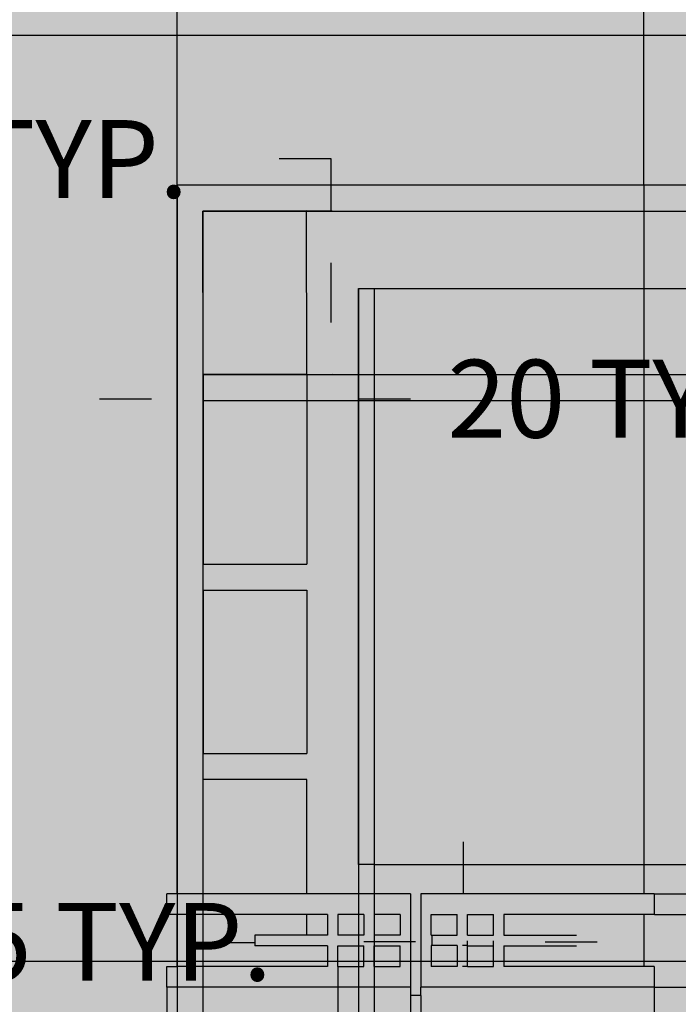
# Model space of a CAD drawing. Units: millimetres. Extents: x 131 to 845, y -20 to 1043.
# Tile 7 of 11: x 495 to 622, y 302 to 492. Entities that reach past the tile are written whole.
import ezdxf

# ---------------------------------------------------------------- set-up
doc = ezdxf.new("R2010")
doc.units = ezdxf.units.MM
doc.header["$MEASUREMENT"] = 0
for name, color, linetype, lineweight in [('A-ANNO-DIMS', 2, 'Continuous', 18), ('A-DOOR', 3, 'Continuous', 25), ('A-DOOR-PATT', 45, 'Continuous', 13), ('A-ELEV', 7, 'Continuous', 25), ('A-ELEV-PATT', 7, 'Continuous', 13), ('A-FLOR-HRAL', 6, 'Continuous', 25), ('A-WALL-PATT', 131, 'Continuous', 13)]:
    doc.layers.add(name, color=color, linetype=linetype, lineweight=lineweight)
doc.styles.get("Standard").update_dxf_attribs({"font": 'arial.ttf'})
doc.dimstyles.get("Standard").update_dxf_attribs({"dimtxt": 15, "dimasz": 10, "dimexe": 0.18, "dimexo": 0.0625, "dimgap": 5, "dimtad": 0, "dimtih": 1, "dimtoh": 1, "dimdec": 0, "dimzin": 0, "dimdsep": 46, "dimtxsty": 'Standard', "dimcen": 5, "dimadec": 0, "dimazin": 0, "dimtfac": 1, "dimtdec": 0, "dimtofl": 0, "dimtmove": 0, "dimatfit": 3, "dimfxl": 1, "dimtolj": 1, "dimtzin": 0, "dimarcsym": 0})

# ---------------------------------------------------------------- blocks, each defined once
blk = doc.blocks.new('RAIL-PANEL')
for p, q in [((5, 4), (0, 4)), ((0, 4), (0, 0)), ((5, 4), (5, 0)), ((5, 0), (0, 0))]:
    blk.add_line(p, q)
blk = doc.blocks.new('DOOR-GLASS-PANE')
for p, q in [((0, 0), (0, 31.5)), ((20, 31.5), (0, 31.5)), ((20, 0), (20, 31.5)), ((20, 0), (0, 0))]:
    blk.add_line(p, q)
blk = doc.blocks.new('*D9')
at = {"layer": 'A-ANNO-DIMS', "color": 0, "lineweight": -2, "transparency": 16777216}
for p, q in [((571.05, 313.91), (561.05, 313.91)), ((581.05, 313.22), (581.05, 314.09)), ((586.05, 313.22), (586.05, 314.09)), ((596.05, 313.91), (606.05, 313.91))]:
    blk.add_line(p, q, dxfattribs=at)
at = {"layer": 'A-ANNO-DIMS', "color": 0, "transparency": 16777216}
for points in [[(571.05, 315.58), (571.05, 312.24), (581.05, 313.91)], [(596.05, 315.58), (596.05, 312.24), (586.05, 313.91)]]:
    blk.add_solid(points, dxfattribs=at)
at = {"layer": 'Defpoints', "color": 0, "transparency": 16777216}
for p in [(581.05, 313.91), (581.05, 313.16), (586.05, 313.16)]:
    blk.add_point(p, dxfattribs=at)
at = {"layer": 'A-ANNO-DIMS', "color": 0, "transparency": 16777216, "insert": (409.24, 313.91), "char_height": 15, "attachment_point": 5}
blk.add_mtext('\\A1;BALCONY RAIL PANEL 5 TYP.', dxfattribs=at)
blk = doc.blocks.new('*D10')
at = {"layer": 'A-ANNO-DIMS', "color": 0, "lineweight": -2, "transparency": 16777216}
for p, q in [((580.3, 323.16), (580.3, 333.16)), ((580.98, 313.16), (580.12, 313.16)), ((580.98, 309.16), (580.12, 309.16)), ((580.3, 299.16), (580.3, 289.16)), ((580.3, 289.16), (570.3, 289.16))]:
    blk.add_line(p, q, dxfattribs=at)
at = {"layer": 'A-ANNO-DIMS', "color": 0, "transparency": 16777216}
for points in [[(578.63, 323.16), (581.96, 323.16), (580.3, 313.16)], [(578.63, 299.16), (581.96, 299.16), (580.3, 309.16)]]:
    blk.add_solid(points, dxfattribs=at)
at = {"layer": 'Defpoints', "color": 0, "transparency": 16777216}
for p in [(581.05, 313.16), (580.3, 309.16), (581.05, 309.16)]:
    blk.add_point(p, dxfattribs=at)
at = {"layer": 'A-ANNO-DIMS', "color": 0, "transparency": 16777216, "insert": (534.31, 289.16), "char_height": 15, "attachment_point": 5}
blk.add_mtext('\\A1;4 TYP.', dxfattribs=at)
blk = doc.blocks.new('*D11')
at = {"layer": 'A-ANNO-DIMS', "color": 0, "lineweight": -2, "transparency": 16777216}
for p, q in [((554.73, 464.78), (544.73, 464.78)), ((554.75, 454.78), (554.73, 464.78)), ((550.09, 454.77), (554.93, 454.78)), ((554.78, 433.28), (554.76, 444.78)), ((550.13, 423.27), (554.97, 423.28))]:
    blk.add_line(p, q, dxfattribs=at)
at = {"layer": 'A-ANNO-DIMS', "color": 0, "transparency": 16777216}
for points in [[(556.43, 444.78), (553.1, 444.77), (554.75, 454.78)], [(556.45, 433.28), (553.11, 433.27), (554.79, 423.28)]]:
    blk.add_solid(points, dxfattribs=at)
at = {"layer": 'Defpoints', "color": 0, "transparency": 16777216}
for p in [(550.02, 454.77), (554.75, 454.78), (550.07, 423.27)]:
    blk.add_point(p, dxfattribs=at)
at = {"layer": 'A-ANNO-DIMS', "color": 0, "transparency": 16777216, "insert": (399.96, 464.78), "char_height": 15, "attachment_point": 5}
blk.add_mtext('\\A1;DOOR GLASS PANE 32 TYP.', dxfattribs=at)
blk = doc.blocks.new('*D12')
at = {"layer": 'A-ANNO-DIMS', "color": 0, "lineweight": -2, "transparency": 16777216}
for p, q in [((530.07, 423.18), (530.08, 418.34)), ((550.07, 423.21), (550.08, 418.36)), ((520.08, 418.5), (510.08, 418.49)), ((560.08, 418.56), (570.08, 418.57))]:
    blk.add_line(p, q, dxfattribs=at)
at = {"layer": 'A-ANNO-DIMS', "color": 0, "transparency": 16777216}
for points in [[(520.07, 420.17), (520.08, 416.83), (530.08, 418.52)], [(560.07, 420.22), (560.08, 416.89), (550.08, 418.54)]]:
    blk.add_solid(points, dxfattribs=at)
at = {"layer": 'Defpoints', "color": 0, "transparency": 16777216}
for p in [(530.07, 423.24), (550.07, 423.27), (550.08, 418.54)]:
    blk.add_point(p, dxfattribs=at)
at = {"layer": 'A-ANNO-DIMS', "color": 0, "transparency": 16777216, "insert": (611.71, 418.57), "char_height": 15, "attachment_point": 5}
blk.add_mtext('\\A1;20 TYP.', dxfattribs=at)
blk = doc.blocks.new('*D50')
at = {"layer": 'A-ANNO-DIMS', "color": 0, "lineweight": -2, "transparency": 16777216}
for p, q in [((720.6, 488.6), (768.56, 488.6)), ((768.38, 478.6), (768.38, 287.12)), ((768.38, 70.31), (768.38, 261.79)), ((216.3, 60.31), (768.56, 60.31))]:
    blk.add_line(p, q, dxfattribs=at)
at = {"layer": 'A-ANNO-DIMS', "color": 0, "transparency": 16777216}
for points in [[(766.72, 478.6), (770.05, 478.6), (768.38, 488.6)], [(766.72, 70.31), (770.05, 70.31), (768.38, 60.31)]]:
    blk.add_solid(points, dxfattribs=at)
at = {"layer": 'Defpoints', "color": 0, "transparency": 16777216}
for p in [(720.53, 488.6), (768.38, 488.6), (216.23, 60.31)]:
    blk.add_point(p, dxfattribs=at)
at = {"layer": 'A-ANNO-DIMS', "color": 0, "transparency": 16777216, "insert": (768.38, 274.45), "char_height": 15, "attachment_point": 5}
blk.add_mtext('\\A1;428.3', dxfattribs=at)
blk = doc.blocks.new('*D51')
at = {"layer": 'A-ANNO-DIMS', "color": 0, "lineweight": -2, "transparency": 16777216}
for p, q in [((658.81, 488.53), (658.81, -10.22)), ((628.88, 312.6), (628.88, -10.22)), ((618.88, -10.04), (608.88, -10.04)), ((668.81, -10.04), (678.81, -10.04))]:
    blk.add_line(p, q, dxfattribs=at)
at = {"layer": 'A-ANNO-DIMS', "color": 0, "transparency": 16777216}
for points in [[(618.88, -8.37), (618.88, -11.7), (628.88, -10.04)], [(668.81, -8.37), (668.81, -11.7), (658.81, -10.04)]]:
    blk.add_solid(points, dxfattribs=at)
at = {"layer": 'Defpoints', "color": 0, "transparency": 16777216}
for p in [(658.81, 488.6), (628.88, 312.66), (658.81, -10.04)]:
    blk.add_point(p, dxfattribs=at)
at = {"layer": 'A-ANNO-DIMS', "color": 0, "transparency": 16777216, "insert": (715.07, -10.04), "char_height": 15, "attachment_point": 5}
blk.add_mtext('\\A1;29.923', dxfattribs=at)
blk = doc.blocks.new('*D58')
at = {"layer": 'A-ANNO-DIMS', "color": 0, "lineweight": -2, "transparency": 16777216}
for p, q in [((525.05, 459.87), (525.05, 1033.7)), ((535.05, 1033.52), (554.33, 1033.52)), ((605.05, 1033.52), (585.76, 1033.52)), ((615.05, 459.87), (615.05, 1033.7))]:
    blk.add_line(p, q, dxfattribs=at)
at = {"layer": 'A-ANNO-DIMS', "color": 0, "transparency": 16777216}
for points in [[(535.05, 1035.18), (535.05, 1031.85), (525.05, 1033.52)], [(605.05, 1035.18), (605.05, 1031.85), (615.05, 1033.52)]]:
    blk.add_solid(points, dxfattribs=at)
at = {"layer": 'Defpoints', "color": 0, "transparency": 16777216}
for p in [(615.05, 1033.52), (525.05, 459.8), (615.05, 459.8)]:
    blk.add_point(p, dxfattribs=at)
at = {"layer": 'A-ANNO-DIMS', "color": 0, "transparency": 16777216, "insert": (570.05, 1033.52), "char_height": 15, "attachment_point": 5}
blk.add_mtext('\\A1;90', dxfattribs=at)
blk = doc.blocks.new('*D59')
at = {"layer": 'A-ANNO-DIMS', "color": 0, "lineweight": -2, "transparency": 16777216}
for p, q in [((615.11, 459.8), (768.56, 459.8)), ((768.38, 449.8), (768.38, 395.14)), ((768.38, 315.16), (768.38, 369.82)), ((617.11, 305.16), (768.56, 305.16))]:
    blk.add_line(p, q, dxfattribs=at)
at = {"layer": 'A-ANNO-DIMS', "color": 0, "transparency": 16777216}
for points in [[(766.72, 449.8), (770.05, 449.8), (768.38, 459.8)], [(766.72, 315.16), (770.05, 315.16), (768.38, 305.16)]]:
    blk.add_solid(points, dxfattribs=at)
at = {"layer": 'Defpoints', "color": 0, "transparency": 16777216}
for p in [(615.05, 459.8), (617.05, 305.16), (768.38, 305.16)]:
    blk.add_point(p, dxfattribs=at)
at = {"layer": 'A-ANNO-DIMS', "color": 0, "transparency": 16777216, "insert": (768.38, 382.48), "char_height": 15, "attachment_point": 5}
blk.add_mtext('\\A1;154.65', dxfattribs=at)
blk = doc.blocks.new('*D60')
at = {"layer": 'A-ANNO-DIMS', "color": 0, "lineweight": -2, "transparency": 16777216}
for p, q in [((768.38, 333.16), (768.38, 343.16)), ((768.38, 343.16), (778.38, 343.16)), ((617.11, 323.16), (768.56, 323.16)), ((617.11, 305.16), (768.56, 305.16)), ((768.38, 295.16), (768.38, 285.16))]:
    blk.add_line(p, q, dxfattribs=at)
at = {"layer": 'A-ANNO-DIMS', "color": 0, "transparency": 16777216}
for points in [[(766.72, 333.16), (770.05, 333.16), (768.38, 323.16)], [(766.72, 295.16), (770.05, 295.16), (768.38, 305.16)]]:
    blk.add_solid(points, dxfattribs=at)
at = {"layer": 'Defpoints', "color": 0, "transparency": 16777216}
for p in [(617.05, 323.16), (768.38, 323.16), (617.05, 305.16)]:
    blk.add_point(p, dxfattribs=at)
at = {"layer": 'A-ANNO-DIMS', "color": 0, "transparency": 16777216, "insert": (793.44, 343.16), "char_height": 15, "attachment_point": 5}
blk.add_mtext('\\A1;18', dxfattribs=at)
blk = doc.blocks.new('*D61')
at = {"layer": 'A-ANNO-DIMS', "color": 0, "lineweight": -2, "transparency": 16777216}
for p, q in [((768.38, 333.16), (768.38, 343.16)), ((768.38, 343.16), (778.38, 343.16)), ((617.11, 323.16), (768.56, 323.16)), ((617.11, 319.16), (768.56, 319.16)), ((768.38, 309.16), (768.38, 299.16))]:
    blk.add_line(p, q, dxfattribs=at)
at = {"layer": 'A-ANNO-DIMS', "color": 0, "transparency": 16777216}
for points in [[(766.72, 333.16), (770.05, 333.16), (768.38, 323.16)], [(766.72, 309.16), (770.05, 309.16), (768.38, 319.16)]]:
    blk.add_solid(points, dxfattribs=at)
at = {"layer": 'Defpoints', "color": 0, "transparency": 16777216}
for p in [(617.05, 323.16), (768.38, 323.16), (617.05, 319.16)]:
    blk.add_point(p, dxfattribs=at)
at = {"layer": 'A-ANNO-DIMS', "color": 0, "transparency": 16777216, "insert": (788.57, 343.16), "char_height": 15, "attachment_point": 5}
blk.add_mtext('\\A1;4', dxfattribs=at)
blk = doc.blocks.new('*D62')
at = {"layer": 'A-ANNO-DIMS', "color": 0, "lineweight": -2, "transparency": 16777216}
for p, q in [((525.05, 459.74), (525.05, -10.22)), ((530.02, 454.68), (530.02, -10.22)), ((515.05, -10.04), (505.05, -10.04)), ((540.02, -10.04), (550.02, -10.04))]:
    blk.add_line(p, q, dxfattribs=at)
at = {"layer": 'A-ANNO-DIMS', "color": 0, "transparency": 16777216}
for points in [[(515.05, -8.37), (515.05, -11.7), (525.05, -10.04)], [(540.02, -8.37), (540.02, -11.7), (530.02, -10.04)]]:
    blk.add_solid(points, dxfattribs=at)
at = {"layer": 'Defpoints', "color": 0, "transparency": 16777216}
for p in [(525.05, 459.8), (530.02, 454.74), (530.02, -10.04)]:
    blk.add_point(p, dxfattribs=at)
at = {"layer": 'A-ANNO-DIMS', "color": 0, "transparency": 16777216, "insert": (580.63, -10.04), "char_height": 15, "attachment_point": 5}
blk.add_mtext('\\A1;4.977', dxfattribs=at)
blk = doc.blocks.new('*D63')
at = {"layer": 'A-ANNO-DIMS', "color": 0, "lineweight": -2, "transparency": 16777216}
for p, q in [((768.38, 469.8), (768.38, 479.8)), ((768.38, 479.8), (778.38, 479.8)), ((525.11, 459.8), (768.56, 459.8)), ((530.09, 454.74), (768.56, 454.74)), ((768.38, 444.74), (768.38, 434.74))]:
    blk.add_line(p, q, dxfattribs=at)
at = {"layer": 'A-ANNO-DIMS', "color": 0, "transparency": 16777216}
for points in [[(766.72, 469.8), (770.05, 469.8), (768.38, 459.8)], [(766.72, 444.74), (770.05, 444.74), (768.38, 454.74)]]:
    blk.add_solid(points, dxfattribs=at)
at = {"layer": 'Defpoints', "color": 0, "transparency": 16777216}
for p in [(525.05, 459.8), (768.38, 459.8), (530.02, 454.74)]:
    blk.add_point(p, dxfattribs=at)
at = {"layer": 'A-ANNO-DIMS', "color": 0, "transparency": 16777216, "insert": (808.75, 479.8), "char_height": 15, "attachment_point": 5}
blk.add_mtext('\\A1;5.065', dxfattribs=at)
blk = doc.blocks.new('*D64')
at = {"layer": 'A-ANNO-DIMS', "color": 0, "lineweight": -2, "transparency": 16777216}
for p, q in [((768.38, 433.24), (768.38, 443.24)), ((768.38, 443.24), (778.38, 443.24)), ((530.13, 423.24), (768.56, 423.24)), ((530.11, 418.2), (768.56, 418.2)), ((768.38, 408.2), (768.38, 398.2))]:
    blk.add_line(p, q, dxfattribs=at)
at = {"layer": 'A-ANNO-DIMS', "color": 0, "transparency": 16777216}
for points in [[(766.72, 433.24), (770.05, 433.24), (768.38, 423.24)], [(766.72, 408.2), (770.05, 408.2), (768.38, 418.2)]]:
    blk.add_solid(points, dxfattribs=at)
at = {"layer": 'Defpoints', "color": 0, "transparency": 16777216}
for p in [(530.07, 423.24), (768.38, 423.24), (530.05, 418.2)]:
    blk.add_point(p, dxfattribs=at)
at = {"layer": 'A-ANNO-DIMS', "color": 0, "transparency": 16777216, "insert": (808.69, 443.24), "char_height": 15, "attachment_point": 5}
blk.add_mtext('\\A1;5.036', dxfattribs=at)
blk = doc.blocks.new('*D65')
at = {"layer": 'A-ANNO-DIMS', "color": 0, "lineweight": -2, "transparency": 16777216}
for p, q in [((560.05, 439.74), (560.05, -10.22)), ((563.05, 439.74), (563.05, -10.22)), ((550.05, -10.04), (540.05, -10.04)), ((573.05, -10.04), (583.05, -10.04))]:
    blk.add_line(p, q, dxfattribs=at)
at = {"layer": 'A-ANNO-DIMS', "color": 0, "transparency": 16777216}
for points in [[(550.05, -8.37), (550.05, -11.7), (560.05, -10.04)], [(573.05, -8.37), (573.05, -11.7), (563.05, -10.04)]]:
    blk.add_solid(points, dxfattribs=at)
at = {"layer": 'Defpoints', "color": 0, "transparency": 16777216}
for p in [(560.05, 439.8), (563.05, 439.8), (563.05, -10.04)]:
    blk.add_point(p, dxfattribs=at)
at = {"layer": 'A-ANNO-DIMS', "color": 0, "transparency": 16777216, "insert": (592.96, -10.04), "char_height": 15, "attachment_point": 5}
blk.add_mtext('\\A1;3', dxfattribs=at)
blk = doc.blocks.new('*D66')
at = {"layer": 'A-ANNO-DIMS', "color": 0, "lineweight": -2, "transparency": 16777216}
for p, q in [((563.11, 439.8), (768.56, 439.8)), ((768.38, 429.8), (768.38, 396.84)), ((768.38, 338.8), (768.38, 371.77)), ((563.11, 328.8), (768.56, 328.8))]:
    blk.add_line(p, q, dxfattribs=at)
at = {"layer": 'A-ANNO-DIMS', "color": 0, "transparency": 16777216}
for points in [[(766.72, 429.8), (770.05, 429.8), (768.38, 439.8)], [(766.72, 338.8), (770.05, 338.8), (768.38, 328.8)]]:
    blk.add_solid(points, dxfattribs=at)
at = {"layer": 'Defpoints', "color": 0, "transparency": 16777216}
for p in [(563.05, 439.8), (768.38, 439.8), (563.05, 328.8)]:
    blk.add_point(p, dxfattribs=at)
at = {"layer": 'A-ANNO-DIMS', "color": 0, "transparency": 16777216, "insert": (768.38, 384.3), "char_height": 15, "attachment_point": 5}
blk.add_mtext('\\A1;111', dxfattribs=at)
blk = doc.blocks.new('*D67')
at = {"layer": 'A-ANNO-DIMS', "color": 0, "lineweight": -2, "transparency": 16777216}
for p, q in [((525.05, 459.74), (525.05, -10.22)), ((560.05, 439.74), (560.05, -10.22)), ((515.05, -10.04), (505.05, -10.04)), ((570.05, -10.04), (580.05, -10.04))]:
    blk.add_line(p, q, dxfattribs=at)
at = {"layer": 'A-ANNO-DIMS', "color": 0, "transparency": 16777216}
for points in [[(515.05, -8.37), (515.05, -11.7), (525.05, -10.04)], [(570.05, -8.37), (570.05, -11.7), (560.05, -10.04)]]:
    blk.add_solid(points, dxfattribs=at)
at = {"layer": 'Defpoints', "color": 0, "transparency": 16777216}
for p in [(525.05, 459.8), (560.05, 439.8), (560.05, -10.04)]:
    blk.add_point(p, dxfattribs=at)
at = {"layer": 'A-ANNO-DIMS', "color": 0, "transparency": 16777216, "insert": (542.55, -10.04), "char_height": 15, "attachment_point": 5}
blk.add_mtext('\\A1;35', dxfattribs=at)
blk = doc.blocks.new('*D68')
at = {"layer": 'A-ANNO-DIMS', "color": 0, "lineweight": -2, "transparency": 16777216}
for p, q in [((523.05, 305.1), (523.05, -10.22)), ((617.05, 305.1), (617.05, -10.22)), ((533.05, -10.04), (554.33, -10.04)), ((607.05, -10.04), (585.76, -10.04))]:
    blk.add_line(p, q, dxfattribs=at)
at = {"layer": 'A-ANNO-DIMS', "color": 0, "transparency": 16777216}
for points in [[(533.05, -8.37), (533.05, -11.7), (523.05, -10.04)], [(607.05, -8.37), (607.05, -11.7), (617.05, -10.04)]]:
    blk.add_solid(points, dxfattribs=at)
at = {"layer": 'Defpoints', "color": 0, "transparency": 16777216}
for p in [(523.05, 305.16), (617.05, 305.16), (617.05, -10.04)]:
    blk.add_point(p, dxfattribs=at)
at = {"layer": 'A-ANNO-DIMS', "color": 0, "transparency": 16777216, "insert": (570.05, -10.04), "char_height": 15, "attachment_point": 5}
blk.add_mtext('\\A1;94', dxfattribs=at)
blk = doc.blocks.new('*D69')
at = {"layer": 'A-ANNO-DIMS', "color": 0, "lineweight": -2, "transparency": 16777216}
for p, q in [((570.05, 303.56), (570.05, -10.22)), ((572.05, 303.56), (572.05, -10.22)), ((560.05, -10.04), (550.05, -10.04)), ((582.05, -10.04), (592.05, -10.04))]:
    blk.add_line(p, q, dxfattribs=at)
at = {"layer": 'A-ANNO-DIMS', "color": 0, "transparency": 16777216}
for points in [[(560.05, -8.37), (560.05, -11.7), (570.05, -10.04)], [(582.05, -8.37), (582.05, -11.7), (572.05, -10.04)]]:
    blk.add_solid(points, dxfattribs=at)
at = {"layer": 'Defpoints', "color": 0, "transparency": 16777216}
for p in [(570.05, 303.62), (572.05, 303.62), (572.05, -10.04)]:
    blk.add_point(p, dxfattribs=at)
at = {"layer": 'A-ANNO-DIMS', "color": 0, "transparency": 16777216, "insert": (616.63, -10.04), "char_height": 15, "attachment_point": 5}
blk.add_mtext('\\A1;2.00', dxfattribs=at)
blk = doc.blocks.new('*D70')
at = {"layer": 'A-ANNO-DIMS', "color": 0, "lineweight": -2, "transparency": 16777216}
for p, q in [((556.05, 309.1), (556.05, -10.22)), ((523.05, 305.1), (523.05, -10.22)), ((513.05, -10.04), (503.05, -10.04)), ((566.05, -10.04), (576.05, -10.04))]:
    blk.add_line(p, q, dxfattribs=at)
at = {"layer": 'A-ANNO-DIMS', "color": 0, "transparency": 16777216}
for points in [[(513.05, -8.37), (513.05, -11.7), (523.05, -10.04)], [(566.05, -8.37), (566.05, -11.7), (556.05, -10.04)]]:
    blk.add_solid(points, dxfattribs=at)
at = {"layer": 'Defpoints', "color": 0, "transparency": 16777216}
for p in [(556.05, 309.16), (523.05, 305.16), (556.05, -10.04)]:
    blk.add_point(p, dxfattribs=at)
at = {"layer": 'A-ANNO-DIMS', "color": 0, "transparency": 16777216, "insert": (539.55, -10.04), "char_height": 15, "attachment_point": 5}
blk.add_mtext('\\A1;33', dxfattribs=at)
blk = doc.blocks.new('*D71')
at = {"layer": 'A-ANNO-DIMS', "color": 0, "lineweight": -2, "transparency": 16777216}
for p, q in [((556.05, 309.1), (556.05, -10.22)), ((563.05, 309.1), (563.05, -10.22)), ((546.05, -10.04), (536.05, -10.04)), ((573.05, -10.04), (583.05, -10.04))]:
    blk.add_line(p, q, dxfattribs=at)
at = {"layer": 'A-ANNO-DIMS', "color": 0, "transparency": 16777216}
for points in [[(546.05, -8.37), (546.05, -11.7), (556.05, -10.04)], [(573.05, -8.37), (573.05, -11.7), (563.05, -10.04)]]:
    blk.add_solid(points, dxfattribs=at)
at = {"layer": 'Defpoints', "color": 0, "transparency": 16777216}
for p in [(556.05, 309.16), (563.05, 309.16), (563.05, -10.04)]:
    blk.add_point(p, dxfattribs=at)
at = {"layer": 'A-ANNO-DIMS', "color": 0, "transparency": 16777216, "insert": (592.9, -10.04), "char_height": 15, "attachment_point": 5}
blk.add_mtext('\\A1;7', dxfattribs=at)
blk = doc.blocks.new('*D75')
at = {"layer": 'A-ANNO-DIMS', "color": 0, "lineweight": -2, "transparency": 16777216}
for p, q in [((462.24, 1033.52), (452.24, 1033.52)), ((472.24, 310.22), (472.24, 1033.7)), ((489.56, 300.22), (489.56, 1033.7)), ((499.56, 1033.52), (509.56, 1033.52))]:
    blk.add_line(p, q, dxfattribs=at)
at = {"layer": 'A-ANNO-DIMS', "color": 0, "transparency": 16777216}
for points in [[(462.24, 1035.18), (462.24, 1031.85), (472.24, 1033.52)], [(499.56, 1035.18), (499.56, 1031.85), (489.56, 1033.52)]]:
    blk.add_solid(points, dxfattribs=at)
at = {"layer": 'Defpoints', "color": 0, "transparency": 16777216}
for p in [(489.56, 1033.52), (472.24, 310.16), (489.56, 300.16)]:
    blk.add_point(p, dxfattribs=at)
at = {"layer": 'A-ANNO-DIMS', "color": 0, "transparency": 16777216, "insert": (539.08, 1033.52), "char_height": 15, "attachment_point": 5}
blk.add_mtext('\\A1;17.32', dxfattribs=at)
blk = doc.blocks.new('*D76')
at = {"layer": 'A-ANNO-DIMS', "color": 0, "lineweight": -2, "transparency": 16777216}
for p, q in [((768.38, 320.16), (768.38, 330.16)), ((472.3, 310.16), (768.56, 310.16)), ((489.62, 300.16), (768.56, 300.16)), ((768.38, 290.16), (768.38, 280.16)), ((768.38, 280.16), (758.38, 280.16))]:
    blk.add_line(p, q, dxfattribs=at)
at = {"layer": 'A-ANNO-DIMS', "color": 0, "transparency": 16777216}
for points in [[(766.72, 320.16), (770.05, 320.16), (768.38, 310.16)], [(766.72, 290.16), (770.05, 290.16), (768.38, 300.16)]]:
    blk.add_solid(points, dxfattribs=at)
at = {"layer": 'Defpoints', "color": 0, "transparency": 16777216}
for p in [(472.24, 310.16), (489.56, 300.16), (768.38, 300.16)]:
    blk.add_point(p, dxfattribs=at)
at = {"layer": 'A-ANNO-DIMS', "color": 0, "transparency": 16777216, "insert": (743.37, 280.16), "char_height": 15, "attachment_point": 5}
blk.add_mtext('\\A1;10', dxfattribs=at)
blk = doc.blocks.new('*D85')
at = {"layer": 'A-ANNO-DIMS', "color": 0, "lineweight": -2, "transparency": 16777216}
for p, q in [((768.38, 301.78), (768.38, 311.78)), ((768.38, 311.78), (778.38, 311.78)), ((639.93, 291.78), (768.56, 291.78)), ((602.06, 283.26), (768.56, 283.26)), ((768.38, 273.26), (768.38, 263.26))]:
    blk.add_line(p, q, dxfattribs=at)
at = {"layer": 'A-ANNO-DIMS', "color": 0, "transparency": 16777216}
for points in [[(766.72, 301.78), (770.05, 301.78), (768.38, 291.78)], [(766.72, 273.26), (770.05, 273.26), (768.38, 283.26)]]:
    blk.add_solid(points, dxfattribs=at)
at = {"layer": 'Defpoints', "color": 0, "transparency": 16777216}
for p in [(639.87, 291.78), (768.38, 291.78), (601.99, 283.26)]:
    blk.add_point(p, dxfattribs=at)
at = {"layer": 'A-ANNO-DIMS', "color": 0, "transparency": 16777216, "insert": (808.63, 311.78), "char_height": 15, "attachment_point": 5}
blk.add_mtext('\\A1;8.522', dxfattribs=at)

msp = doc.modelspace()

# ---------------------------------------------------------------- hatches: boundary and pattern name
at = {"layer": 'A-DOOR-PATT'}
h = msp.add_hatch(color=256, dxfattribs=at)
h.dxf.hatch_style = 1
h.paths.add_polyline_path([(615.0467, 459.8046), (525.0467, 459.8046), (525.0467, 323.1596), (530.0467, 323.1596), (530.0467, 345.2044), (550.0467, 345.2044), (550.0467, 323.1596), (570.0467, 323.1596), (570.0467, 305.1596), (570.0467, 303.6234), (572.0453, 303.6234), (572.0467, 305.1596), (572.0467, 323.1596), (615.0467, 323.1596)])
h.paths.add_polyline_path([(563.0467, 328.8046), (560.0467, 328.8046), (560.0467, 439.8046), (563.0467, 439.8046)], flags=16)
h.paths.add_polyline_path([(550.0467, 386.7044), (530.0467, 386.7044), (530.0467, 418.2044), (550.0467, 418.2044)], flags=16)
h.paths.add_polyline_path([(550.0467, 381.7044), (550.0467, 350.2044), (530.0467, 350.2044), (530.0467, 381.7044)], flags=16)
h.paths.add_polyline_path([(550.0467, 423.2044), (530.0467, 423.2044), (530.0467, 454.8046), (550.0467, 454.8046)], flags=16)
h.paths.add_polyline_path([(615.0467, 693.2667), (525.0467, 693.2667), (525.0467, 542.1664), (615.0467, 542.1664)])
h.paths.add_polyline_path([(563.0467, 562.2667), (560.0467, 562.2667), (560.0467, 673.2667), (563.0467, 673.2667)], flags=16)
h.paths.add_polyline_path([(550.0467, 583.6664), (530.0467, 583.6664), (530.0467, 615.1664), (550.0467, 615.1664)], flags=16)
h.paths.add_polyline_path([(550.0467, 578.6664), (550.0467, 547.1664), (530.0467, 547.1664), (530.0467, 578.6664)], flags=16)
h.paths.add_polyline_path([(550.0467, 620.1664), (530.0467, 620.1664), (530.0467, 651.6664), (550.0467, 651.6664)], flags=16)
h.paths.add_polyline_path([(550.0467, 656.6664), (530.0467, 656.6664), (530.0467, 688.2667), (550.0467, 688.2667)], flags=16)
h = msp.add_hatch(color=256, dxfattribs=at)
h.dxf.hatch_style = 1
h.paths.add_polyline_path([(523.0467, 323.1596), (523.0467, 319.1596), (525.0467, 319.1596), (554.0467, 319.1596), (554.0467, 315.1596), (540.0467, 315.1596), (540.0467, 313.1596), (554.0467, 313.1596), (554.0467, 309.1596), (525.0467, 309.1596), (523.0467, 309.1596), (523.0467, 305.1596), (525.0467, 305.1596), (570.0467, 305.1596), (570.0467, 323.1596)])
h.paths.add_polyline_path([(556.0467, 319.1596), (561.0467, 319.1596), (561.0467, 315.1596), (556.0467, 315.1596)], flags=16)
h.paths.add_polyline_path([(556.0467, 313.1596), (561.0467, 313.1596), (561.0467, 309.1596), (556.0467, 309.1596)], flags=16)
h.paths.add_polyline_path([(563.0467, 319.1596), (568.0467, 319.1596), (568.0467, 315.1596), (563.0467, 315.1596)], flags=16)
h.paths.add_polyline_path([(563.0467, 313.1596), (568.0467, 313.1596), (568.0467, 309.1596), (563.0467, 309.1596)], flags=16)
h.paths.add_polyline_path([(572.0467, 323.1596), (572.0467, 305.1596), (617.0467, 305.1596), (617.0467, 309.1596), (588.0467, 309.1596), (588.0467, 313.1596), (602.0467, 313.1596), (602.0467, 315.1596), (588.0467, 315.1596), (588.0467, 319.1596), (617.0467, 319.1596), (617.0467, 323.1596)])
h.paths.add_polyline_path([(581.0467, 319.1596), (586.0467, 319.1596), (586.0467, 315.1596), (581.0467, 315.1596)], flags=16)
h.paths.add_polyline_path([(579.0467, 319.1596), (579.0467, 315.1596), (574.0467, 315.1596), (574.0467, 319.1596)], flags=16)
h.paths.add_polyline_path([(581.0467, 313.1596), (586.0467, 313.1596), (586.0467, 309.1596), (581.0467, 309.1596)], flags=16)
h.paths.add_polyline_path([(579.0467, 313.1596), (579.0467, 309.1596), (574.0467, 309.1596), (574.0467, 313.1596)], flags=16)
at = {"layer": 'A-ELEV-PATT', "transparency": 33554681}
h = msp.add_hatch(color=256, dxfattribs=at)
h.set_gradient(color1=(99, 100, 102), color2=(199, 200, 202), name='SPHERICAL')
h.paths.add_polyline_path([(550.0467, 688.2667), (530.0467, 688.2667), (530.0467, 656.6664), (550.0467, 656.6664)])
h.paths.add_polyline_path([(530.0467, 620.1664), (550.0467, 620.1664), (550.0467, 651.6664), (530.0467, 651.6664)])
h.paths.add_polyline_path([(550.0467, 615.1664), (530.0467, 615.1664), (530.0467, 583.6664), (550.0467, 583.6664)])
h.paths.add_polyline_path([(550.0467, 547.1664), (550.0467, 578.6664), (530.0467, 578.6664), (530.0467, 547.1664)])
h.paths.add_polyline_path([(563.0467, 673.2667), (560.0467, 673.2667), (560.0467, 562.2667), (563.0467, 562.2667)])
h.paths.add_polyline_path([(550.0467, 423.2044), (550.0467, 454.8046), (530.0467, 454.8046), (530.0467, 423.2044)])
h.paths.add_polyline_path([(550.0467, 418.2044), (530.0467, 418.2044), (530.0467, 386.7044), (550.0467, 386.7044)])
h.paths.add_polyline_path([(530.0467, 350.2044), (550.0467, 350.2044), (550.0467, 381.7044), (530.0467, 381.7044)])
h.paths.add_polyline_path([(550.0467, 323.1596), (550.0467, 345.2044), (530.0467, 345.2044), (530.0467, 323.1596)])
h.paths.add_polyline_path([(563.0467, 439.8046), (560.0467, 439.8046), (560.0467, 328.8046), (563.0467, 328.8046)])
h = msp.add_hatch(color=256, dxfattribs=at)
h.set_gradient(color1=(255, 255, 255), color2=(199, 200, 202), name='INVSPHERICAL')
h.paths.add_polyline_path([(459.5586, 310.1596), (472.2381, 310.1596), (489.5586, 300.1596), (650.5349, 300.1596), (628.8842, 312.6596), (628.8842, 488.5953), (459.5586, 488.5953)])
h.paths.add_polyline_path([(525.0467, 459.8046), (615.0467, 459.8046), (615.0467, 323.1596), (617.0467, 323.1596), (617.0467, 319.1596), (615.0467, 319.1596), (615.0467, 309.1596), (617.0467, 309.1596), (617.0467, 305.1596), (572.0467, 305.1596), (572.0453, 303.6234), (570.0467, 303.6234), (570.0467, 305.1596), (525.0467, 305.1596), (523.0467, 305.1596), (523.0467, 309.1596), (525.0467, 309.1596), (525.0467, 319.1596), (523.0467, 319.1596), (523.0467, 323.1596), (525.0467, 323.1596)], flags=16)
h.paths.add_polyline_path([(530.0467, 454.8046), (550.0467, 454.8046), (550.0467, 423.2044), (530.0467, 423.2044)], flags=0)
h.paths.add_polyline_path([(530.0467, 418.2044), (550.0467, 418.2044), (550.0467, 386.7044), (530.0467, 386.7044)], flags=0)
h.paths.add_polyline_path([(560.0467, 439.8046), (563.0467, 439.8046), (563.0467, 328.8046), (560.0467, 328.8046)], flags=0)
h.paths.add_polyline_path([(530.0467, 381.7044), (550.0467, 381.7044), (550.0467, 350.2044), (530.0467, 350.2044)], flags=0)
h.paths.add_polyline_path([(554.0467, 319.1596), (554.0467, 315.1596), (540.0467, 315.1596), (540.0467, 313.7044), (530.0467, 313.7044), (530.0467, 319.1596)], flags=0)
h.paths.add_polyline_path([(556.0467, 319.1596), (561.0467, 319.1596), (561.0467, 315.1596), (556.0467, 315.1596)], flags=0)
h.paths.add_polyline_path([(563.0467, 319.1596), (568.0467, 319.1596), (568.0467, 315.1596), (563.0467, 315.1596)], flags=0)
h.paths.add_polyline_path([(556.0467, 313.1596), (561.0467, 313.1596), (561.0467, 309.1596), (556.0467, 309.1596)], flags=0)
h.paths.add_polyline_path([(563.0467, 313.1596), (568.0467, 313.1596), (568.0467, 309.1596), (563.0467, 309.1596)], flags=0)
h.paths.add_polyline_path([(574.0467, 319.1596), (579.0467, 319.1596), (579.0467, 315.1596), (574.1854, 315.1596), (574.1854, 313.1596), (579.0467, 313.1596), (579.0467, 309.1596), (574.0467, 309.1596), (574.0467, 313.1596), (574.1854, 315.1596), (574.0467, 315.1596)], flags=0)
h.paths.add_polyline_path([(581.0467, 319.1596), (586.0467, 319.1596), (586.0467, 315.1596), (581.0467, 315.1596)], flags=0)
h.paths.add_polyline_path([(581.0467, 313.1596), (586.0467, 313.1596), (586.0467, 309.1596), (581.0467, 309.1596)], flags=0)
h = msp.add_hatch(color=256, dxfattribs=at)
h.set_gradient(color1=(79, 2, 22), color2=(98, 46, 19), name='SPHERICAL')
h.paths.add_polyline_path([(615.0467, 459.8046), (525.0467, 459.8046), (525.0467, 323.1596), (530.0467, 323.1596), (530.0467, 345.2044), (550.0467, 345.2044), (550.0467, 323.1596), (570.0467, 323.1596), (570.0467, 305.1596), (570.0467, 303.6234), (572.0453, 303.6234), (572.0467, 305.1596), (572.0467, 323.1596), (615.0467, 323.1596)])
h.paths.add_polyline_path([(563.0467, 328.8046), (560.0467, 328.8046), (560.0467, 439.8046), (563.0467, 439.8046)], flags=16)
h.paths.add_polyline_path([(550.0467, 386.7044), (530.0467, 386.7044), (530.0467, 418.2044), (550.0467, 418.2044)], flags=16)
h.paths.add_polyline_path([(550.0467, 381.7044), (550.0467, 350.2044), (530.0467, 350.2044), (530.0467, 381.7044)], flags=16)
h.paths.add_polyline_path([(550.0467, 423.2044), (530.0467, 423.2044), (530.0467, 454.8046), (550.0467, 454.8046)], flags=16)
h = msp.add_hatch(color=256, dxfattribs=at)
h.set_gradient(color1=(79, 2, 22), color2=(126, 16, 40), name='INVSPHERICAL')
h.paths.add_polyline_path([(615.0467, 309.1596), (615.0467, 319.1596), (617.0467, 319.1596), (617.0467, 323.1596), (572.0467, 323.1596), (572.0467, 305.1596), (617.0467, 305.1596), (617.0467, 309.1596)])
h.paths.add_polyline_path([(586.0467, 309.1596), (581.0467, 309.1596), (581.0467, 313.1596), (586.0467, 313.1596)], flags=16)
h.paths.add_polyline_path([(586.0467, 315.1596), (581.0467, 315.1596), (581.0467, 319.1596), (586.0467, 319.1596)], flags=16)
h.paths.add_polyline_path([(579.0467, 309.1596), (574.0467, 309.1596), (574.0467, 313.1596), (574.1854, 313.1596), (574.1854, 315.1596), (574.0467, 315.1596), (574.0467, 319.1596), (579.0467, 319.1596), (579.0467, 315.1596), (574.1854, 315.1596), (574.1854, 313.1596), (579.0467, 313.1596)], flags=16)
h = msp.add_hatch(color=256, dxfattribs=at)
h.set_gradient(color1=(79, 2, 22), color2=(126, 16, 40), name='INVSPHERICAL')
h.paths.add_polyline_path([(530.0467, 313.7044), (530.0467, 319.1596), (525.0467, 319.1596), (525.0467, 309.1596), (554.0467, 309.1596), (554.0467, 313.1596), (540.0467, 313.1596), (540.0467, 313.7044)])
at = {"layer": 'A-WALL-PATT'}
h = msp.add_hatch(color=256, dxfattribs=at)
h.dxf.hatch_style = 1
h.paths.add_polyline_path([(449.5586, 833.5953), (451.6297, 835.6663), (451.6297, 885.6663), (466.6297, 885.6663), (466.6297, 891.3345), (330.6595, 891.3345), (330.6595, 856.8345), (292.1595, 856.8345), (292.1595, 798.4332), (336.1595, 798.4332), (336.1595, 178.4332), (246.1595, 178.4332), (246.1595, 798.4332), (290.1595, 798.4332), (290.1595, 856.8345), (259.6595, 856.8345), (255.6595, 860.8345), (255.6595, 927.8345), (290.1595, 927.8345), (290.1595, 960.6663), (216.2327, 960.6663), (216.2327, 60.3131), (459.5586, 60.3131), (459.5586, 97.8131), (459.5586, 252.07), (459.5586, 283.5561), (369.5586, 283.5561), (369.5586, 763.5561), (439.5586, 763.5561), (439.5586, 778.6714), (439.5586, 793.5953), (439.5586, 796.5953), (441.5586, 798.5953), (444.5586, 798.5953), (444.5586, 813.5953), (444.5586, 816.5953), (446.5586, 818.5953), (449.5586, 818.5953)])
h.paths.add_polyline_path([(466.6297, 960.6663), (292.1595, 960.6663), (292.1595, 927.8345), (326.6595, 927.8345), (330.6595, 923.8345), (330.6595, 893.3345), (466.6297, 893.3345)], flags=17)
h.paths.add_polyline_path([(720.5349, 813.5953), (720.5349, 818.5953), (710.5349, 818.5953), (449.5586, 818.5953), (446.5586, 818.5953), (444.5586, 816.5953), (444.5586, 813.5953), (444.5586, 798.5953), (705.5349, 798.5953), (705.5349, 513.5953), (705.5349, 498.5953), (680.5349, 498.5953), (680.5349, 488.5953), (705.5349, 488.5953), (720.5349, 488.5953), (720.5349, 513.5953)])
h.paths.add_polyline_path([(680.5349, 498.5953), (412.6606, 498.5953), (412.6606, 488.5953), (680.5349, 488.5953)])

# ---------------------------------------------------------------- linework, layer by layer
at = {"layer": 'A-DOOR'}
for p, q in [((525.0467, 459.8046), (615.0467, 459.8046)), ((525.0467, 323.1596), (525.0467, 459.8046)), ((615.0467, 459.8046), (615.0467, 323.1596)), ((550.0467, 345.2044), (530.0467, 345.2044)), ((530.0467, 323.1596), (530.0467, 345.2044)), ((550.0467, 323.1596), (550.0467, 345.2044)), ((570.0467, 305.1596), (570.0467, 303.6234)), ((570.0467, 303.6234), (572.0453, 303.6234)), ((572.0453, 303.6234), (572.0467, 305.1596))]:
    msp.add_line(p, q, dxfattribs=at)
msp.add_lwpolyline([(560.0467, 439.8046), (563.0467, 439.8046), (563.0467, 328.8046), (560.0467, 328.8046)], close=True, dxfattribs=at)
at = {"layer": 'A-ELEV'}
msp.add_line((705.5349, 488.5953), (412.6606, 488.5953), dxfattribs=at)
at = {"layer": 'A-FLOR-HRAL'}
for p, q in [((523.0467, 319.1596), (523.0467, 323.1596)), ((570.0467, 323.1596), (523.0467, 323.1596)), ((570.0467, 323.1596), (570.0467, 305.1596)), ((617.0467, 323.1596), (572.0467, 323.1596)), ((572.0467, 323.1596), (572.0467, 305.1596)), ((617.0467, 323.1596), (617.0467, 319.1596)), ((525.0467, 319.1596), (523.0467, 319.1596)), ((525.0467, 309.1596), (525.0467, 319.1596)), ((554.0467, 319.1596), (525.0467, 319.1596)), ((530.0467, 313.7044), (530.0467, 319.1596)), ((550.0467, 315.1596), (550.0467, 319.1596)), ((554.0467, 319.1596), (554.0467, 315.1596)), ((617.0467, 319.1596), (588.0467, 319.1596)), ((588.0467, 319.1596), (588.0467, 315.1596)), ((615.0467, 319.1596), (615.0467, 309.1596)), ((540.0467, 315.1596), (540.0467, 313.1596)), ((554.0467, 315.1596), (540.0467, 315.1596)), ((574.1854, 315.1596), (574.1854, 313.1596)), ((588.0467, 315.1596), (602.0467, 315.1596)), ((540.0467, 313.7044), (530.0467, 313.7044)), ((554.0467, 313.1596), (540.0467, 313.1596)), ((554.0467, 313.1596), (554.0467, 309.1596)), ((588.0467, 313.1596), (588.0467, 309.1596)), ((588.0467, 313.1596), (602.0467, 313.1596)), ((523.0467, 305.1596), (523.0467, 309.1596)), ((523.0467, 309.1596), (525.0467, 309.1596)), ((554.0467, 309.1596), (525.0467, 309.1596)), ((617.0467, 309.1596), (588.0467, 309.1596)), ((617.0467, 309.1596), (617.0467, 305.1596)), ((525.0467, 305.1596), (523.0467, 305.1596)), ((570.0467, 305.1596), (525.0467, 305.1596)), ((617.0467, 305.1596), (572.0467, 305.1596))]:
    msp.add_line(p, q, dxfattribs=at)

# ---------------------------------------------------------------- block references
at = {"layer": 'A-DOOR'}
for p, rotation in [((530.0696, 423.2398), 0.0823557908083867), ((550.0465, 418.2047), 180), ((550.0465, 381.7047), 180)]:
    msp.add_blockref('DOOR-GLASS-PANE', p, dxfattribs=dict(at, rotation=rotation))
at = {"layer": 'A-FLOR-HRAL'}
for p in [(556.047, 315.16), (563.047, 315.16), (574.047, 309.16)]:
    msp.add_blockref('RAIL-PANEL', p, dxfattribs=at)
at = {"layer": 'A-FLOR-HRAL', "rotation": 180}
for p in [(579.0465, 319.1592), (586.0465, 319.1592), (561.0465, 313.1592), (568.0465, 313.1592), (586.0465, 313.1592)]:
    msp.add_blockref('RAIL-PANEL', p, dxfattribs=at)

# ---------------------------------------------------------------- dimensions: what is measured, and where the dimension line sits
at = {"layer": 'A-ANNO-DIMS'}
for base, p1, p2, override, picture, middle in [((489.5586, 1033.5163), (472.2381, 310.1596), (489.5586, 300.1596), {"dimdec": 2, "dimlfac": 1, "dimrnd": 0, "dimzin": 0, "dimdsep": 46, "dimlunit": 2}, '*D75', (539.0845, 1033.5163)), ((615.0467, 1033.5163), (525.0467, 459.8046), (615.0467, 459.8046), {"dimdec": 0, "dimlfac": 1, "dimrnd": 0, "dimzin": 0, "dimdsep": 46, "dimlunit": 2}, '*D58', (570.0467, 1033.5163)), ((658.8074, -10.0369), (628.8842, 312.6596), (658.8074, 488.5953), {"dimdec": 3, "dimlfac": 1, "dimrnd": 0, "dimzin": 0, "dimdsep": 46, "dimlunit": 2}, '*D51', (715.0711, -10.0369)), ((530.0241, -10.0369), (525.0467, 459.8046), (530.0241, 454.7401), {"dimdec": 3, "dimlfac": 1, "dimrnd": 0, "dimzin": 0, "dimdsep": 46, "dimlunit": 2}, '*D62', (580.6346, -10.0369)), ((560.0467, -10.0369), (525.0467, 459.8046), (560.0467, 439.8046), {"dimdec": 0, "dimlfac": 1, "dimrnd": 0, "dimzin": 0, "dimdsep": 46, "dimlunit": 2}, '*D67', (542.5467, -10.0369)), ((563.0467, -10.0369), (560.0467, 439.8046), (563.0467, 439.8046), {"dimdec": 0, "dimlfac": 1, "dimrnd": 0, "dimzin": 0, "dimdsep": 46, "dimlunit": 2}, '*D65', (592.9581, -10.0369)), ((556.0467, -10.0369), (523.0467, 305.1596), (556.0467, 309.1596), {"dimdec": 0, "dimlfac": 1, "dimrnd": 0, "dimzin": 0, "dimdsep": 46, "dimlunit": 2}, '*D70', (539.5467, -10.0369)), ((563.0467, -10.0369), (556.0467, 309.1596), (563.0467, 309.1596), {"dimdec": 0, "dimlfac": 1, "dimrnd": 0, "dimzin": 0, "dimdsep": 46, "dimlunit": 2}, '*D71', (592.9018, -10.0369)), ((617.0467, -10.0369), (523.0467, 305.1596), (617.0467, 305.1596), {"dimdec": 0, "dimlfac": 1, "dimrnd": 0, "dimzin": 0, "dimdsep": 46, "dimlunit": 2}, '*D68', (570.0467, -10.0369)), ((572.0453, -10.0369), (570.0467, 303.6234), (572.0453, 303.6234), {"dimdec": 2, "dimlfac": 1, "dimrnd": 0, "dimzin": 0, "dimdsep": 46, "dimlunit": 2}, '*D69', (616.6292, -10.0369))]:
    dim = msp.add_linear_dim(base=base, p1=p1, p2=p2, dimstyle='Standard', override=override, dxfattribs=at)
    dim.commit()
    dim.dimension.update_dxf_attribs({"geometry": picture, "text_midpoint": middle})
for base, p1, p2, angle, text, picture, middle in [((554.7491, 454.7757), (550.0694, 423.2689), (550.0241, 454.7689), 90.082356, 'DOOR GLASS PANE <> TYP.', '*D11', (399.9615, 464.7756)), ((550.0762, 418.5439), (530.0694, 423.2401), (550.0694, 423.2689), 0.082356, '<> TYP.', '*D12', (611.7115, 418.5726)), ((581.0467, 313.9096), (586.0467, 313.1596), (581.0467, 313.1596), 180, 'BALCONY RAIL PANEL <> TYP.', '*D9', (409.2391, 313.9096)), ((580.2967, 309.1596), (581.0467, 313.1596), (581.0467, 309.1596), 270, '<> TYP.', '*D10', (534.3145, 289.1596))]:
    dim = msp.add_linear_dim(base=base, p1=p1, p2=p2, angle=angle, text=text, dimstyle='Standard', override={"dimdec": 0, "dimrnd": 0, "dimzin": 0, "dimlunit": 2}, dxfattribs=at)
    dim.commit()
    dim.dimension.update_dxf_attribs({"geometry": picture, "text_midpoint": middle})
for base, p1, p2, override, picture, middle in [((768.38488, 459.80465), (530.0241, 454.74011), (525.04673, 459.80464), {"dimdec": 3, "dimlfac": 1, "dimrnd": 0, "dimzin": 0, "dimdsep": 46, "dimlunit": 2}, '*D63', (808.74982, 479.80464)), ((768.3849, 488.5953), (216.2327, 60.3131), (720.5349, 488.5953), {"dimdec": 1, "dimlfac": 1, "dimrnd": 0, "dimzin": 0, "dimdsep": 46, "dimlunit": 2}, '*D50', (768.3849, 274.4542)), ((768.38488, 305.1596), (615.04673, 459.80464), (617.04673, 305.1596), {"dimdec": 2, "dimlfac": 1, "dimrnd": 0, "dimzin": 0, "dimdsep": 46, "dimlunit": 2}, '*D59', (768.38488, 382.48212)), ((768.3849, 423.2401), (530.0467, 418.2044), (530.0694, 423.2401), {"dimdec": 3, "dimlfac": 1, "dimrnd": 0, "dimzin": 0, "dimdsep": 46, "dimlunit": 2}, '*D64', (808.6884, 443.2401)), ((768.3849, 439.8046), (563.0467, 328.8046), (563.0467, 439.8046), {"dimdec": 0, "dimlfac": 1, "dimrnd": 0, "dimzin": 0, "dimdsep": 46, "dimlunit": 2}, '*D66', (768.3849, 384.3046)), ((768.3849, 323.1596), (617.0467, 305.1596), (617.0467, 323.1596), {"dimdec": 0, "dimlfac": 1, "dimrnd": 0, "dimzin": 0, "dimdsep": 46, "dimlunit": 2}, '*D60', (793.4377, 343.1596)), ((768.3849, 323.1596), (617.0467, 319.1596), (617.0467, 323.1596), {"dimdec": 0, "dimlfac": 1, "dimrnd": 0, "dimzin": 0, "dimdsep": 46, "dimlunit": 2}, '*D61', (788.5725, 343.1596)), ((768.3849, 300.1596), (472.2381, 310.1596), (489.5586, 300.1596), {"dimdec": 0, "dimlfac": 1, "dimrnd": 0, "dimzin": 0, "dimdsep": 46, "dimlunit": 2}, '*D76', (743.3729, 280.1596)), ((768.3849, 291.7824), (601.9946, 283.2603), (639.8713, 291.7824), {"dimdec": 3, "dimlfac": 1, "dimrnd": 0, "dimzin": 0, "dimdsep": 46, "dimlunit": 2}, '*D85', (808.627, 311.7824))]:
    dim = msp.add_linear_dim(base=base, p1=p1, p2=p2, angle=90, dimstyle='Standard', override=override, dxfattribs=at)
    dim.commit()
    dim.dimension.update_dxf_attribs({"geometry": picture, "text_midpoint": middle})

doc.saveas('drawing.dxf')
